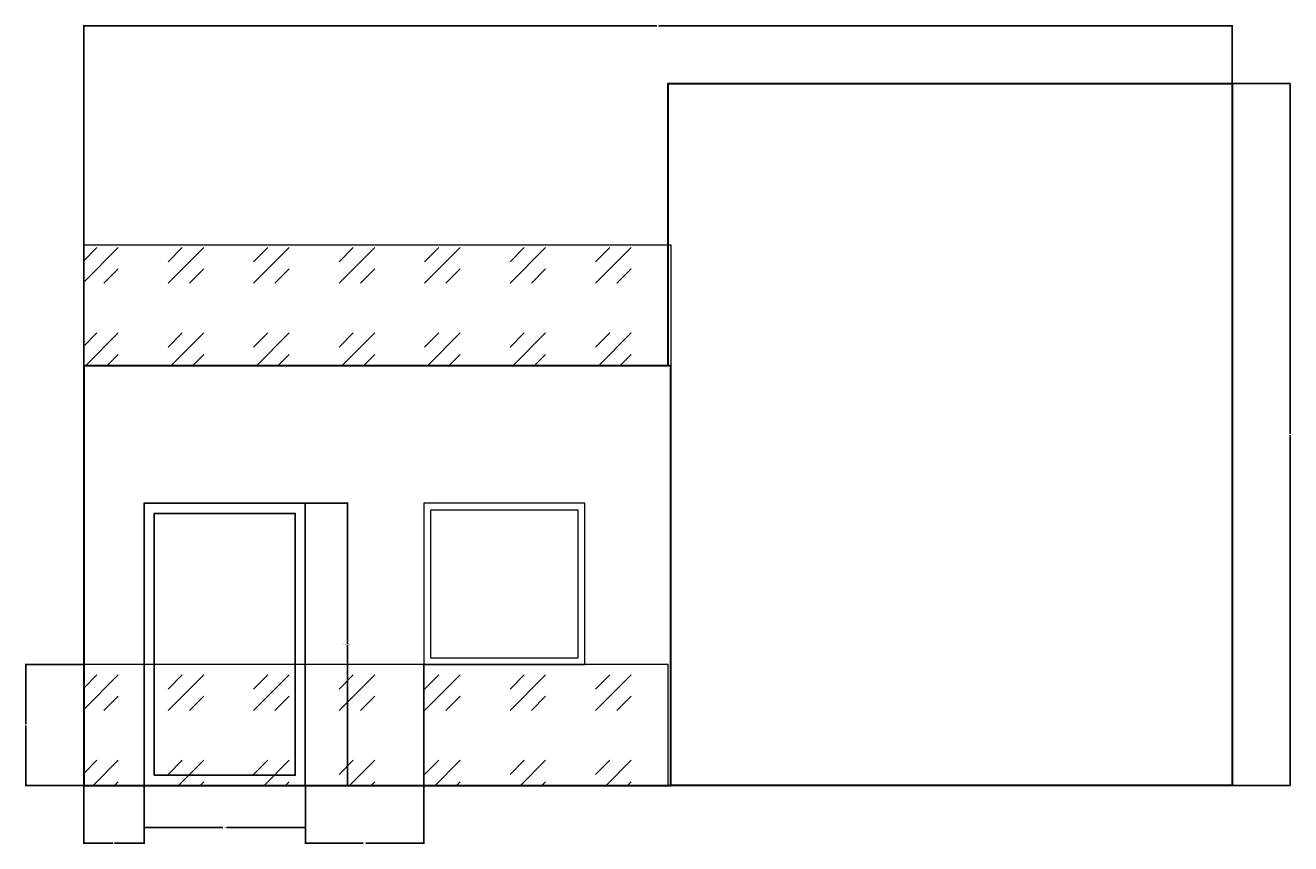
# Model space of a CAD drawing. Units: inches. Extents: x 810 to 2232, y 728 to 1827.
# Tile 3 of 6: x 1841 to 2218, y 749 to 993. Entities that reach past the tile are written whole.
import ezdxf

# ---------------------------------------------------------------- set-up
doc = ezdxf.new("R2010")
doc.units = ezdxf.units.IN
for name, color, linetype, lineweight in [('A-ANNO-DIMS', 2, 'Continuous', 18), ('A-ELEV', 7, 'Continuous', 30), ('A-ELEV-DOOR', 7, 'Continuous', 25), ('A-ELEV-GLAZ', 7, 'Continuous', 18), ('A-ELEV-PATT', 8, 'Continuous', 13)]:
    doc.layers.add(name, color=color, linetype=linetype, lineweight=lineweight)
doc.styles.get("Standard").update_dxf_attribs({"font": 'arial.ttf'})
doc.dimstyles.get("Standard").update_dxf_attribs({"dimtxt": 0.18, "dimasz": 0.18, "dimexe": 0.18, "dimexo": 0.0625, "dimgap": 0.09, "dimtad": 0, "dimtih": 1, "dimtoh": 1, "dimdec": 4, "dimzin": 0, "dimdsep": 46, "dimtxsty": 'Standard', "dimcen": 0.09, "dimadec": 0, "dimazin": 0, "dimtfac": 1, "dimtdec": 4, "dimtofl": 0, "dimtmove": 0, "dimatfit": 3, "dimfxl": 1, "dimtolj": 1, "dimtzin": 0, "dimarcsym": 0})

# ---------------------------------------------------------------- blocks, each defined once
blk = doc.blocks.new('DOOR-BALCONY-ELEV')
for points in [[(0, 0), (48, 0), (48, 84), (0, 84)], [(3, 3), (45, 3), (45, 81), (3, 81)]]:
    blk.add_lwpolyline(points, close=True)
blk = doc.blocks.new('WIN-ELEV-SQUARE')
for points in [[(0, 0), (48, 0), (48, 48), (0, 48)], [(2, 2), (46, 2), (46, 46), (2, 46)]]:
    blk.add_lwpolyline(points, close=True)
blk = doc.blocks.new('*D47')
at = {"layer": 'A-ANNO-DIMS', "color": 0, "lineweight": -2, "transparency": 16777216}
for p, q in [((1924.68, 850.84), (1937.4, 850.84)), ((1937.22, 850.66), (1937.22, 809.02)), ((1937.22, 767.02), (1937.22, 808.66)), ((1924.68, 766.84), (1937.4, 766.84))]:
    blk.add_line(p, q, dxfattribs=at)
at = {"layer": 'A-ANNO-DIMS', "color": 0, "transparency": 16777216}
for points in [[(1937.19, 850.66), (1937.25, 850.66), (1937.22, 850.84)], [(1937.19, 767.02), (1937.25, 767.02), (1937.22, 766.84)]]:
    blk.add_solid(points, dxfattribs=at)
at = {"layer": 'Defpoints', "color": 0, "transparency": 16777216}
for p in [(1924.62, 850.84), (1937.22, 850.84), (1924.62, 766.84)]:
    blk.add_point(p, dxfattribs=at)
at = {"layer": 'A-ANNO-DIMS', "color": 0, "transparency": 16777216, "insert": (1937.22, 808.84), "char_height": 0.18, "attachment_point": 5}
blk.add_mtext('\\A1;BALCONY DOOR 84 TYP.', dxfattribs=at)
blk = doc.blocks.new('*D48')
at = {"layer": 'A-ANNO-DIMS', "color": 0, "lineweight": -2, "transparency": 16777216}
for p, q in [((1876.62, 766.78), (1876.62, 754.06)), ((1924.62, 766.78), (1924.62, 754.06)), ((1876.8, 754.24), (1900.09, 754.24)), ((1924.44, 754.24), (1901.15, 754.24))]:
    blk.add_line(p, q, dxfattribs=at)
at = {"layer": 'A-ANNO-DIMS', "color": 0, "transparency": 16777216}
for points in [[(1876.8, 754.27), (1876.8, 754.21), (1876.62, 754.24)], [(1924.44, 754.27), (1924.44, 754.21), (1924.62, 754.24)]]:
    blk.add_solid(points, dxfattribs=at)
at = {"layer": 'Defpoints', "color": 0, "transparency": 16777216}
for p in [(1876.62, 766.84), (1924.62, 766.84), (1924.62, 754.24)]:
    blk.add_point(p, dxfattribs=at)
at = {"layer": 'A-ANNO-DIMS', "color": 0, "transparency": 16777216, "insert": (1900.62, 754.24), "char_height": 0.18, "attachment_point": 5}
blk.add_mtext('\\A1;48 TYP.', dxfattribs=at)
blk = doc.blocks.new('*D88')
at = {"layer": 'A-ANNO-DIMS', "color": 0, "lineweight": -2, "transparency": 16777216}
for p, q in [((1858.62, 766.9), (1858.62, 993.22)), ((1858.8, 993.04), (2029.33, 993.04)), ((2200.44, 993.04), (2029.9, 993.04)), ((2200.62, 766.9), (2200.62, 993.22))]:
    blk.add_line(p, q, dxfattribs=at)
at = {"layer": 'A-ANNO-DIMS', "color": 0, "transparency": 16777216}
for points in [[(1858.8, 993.07), (1858.8, 993.01), (1858.62, 993.04)], [(2200.44, 993.07), (2200.44, 993.01), (2200.62, 993.04)]]:
    blk.add_solid(points, dxfattribs=at)
at = {"layer": 'Defpoints', "color": 0, "transparency": 16777216}
for p in [(2200.62, 993.04), (1858.62, 766.84), (2200.62, 766.84)]:
    blk.add_point(p, dxfattribs=at)
at = {"layer": 'A-ANNO-DIMS', "color": 0, "transparency": 16777216, "insert": (2029.62, 993.04), "char_height": 0.18, "attachment_point": 5}
blk.add_mtext('\\A1;342', dxfattribs=at)
blk = doc.blocks.new('*D89')
at = {"layer": 'A-ANNO-DIMS', "color": 0, "lineweight": -2, "transparency": 16777216}
for p, q in [((2200.68, 975.84), (2218, 975.84)), ((2217.82, 975.66), (2217.82, 871.52)), ((2217.82, 767.02), (2217.82, 871.16)), ((2200.68, 766.84), (2218, 766.84))]:
    blk.add_line(p, q, dxfattribs=at)
at = {"layer": 'A-ANNO-DIMS', "color": 0, "transparency": 16777216}
for points in [[(2217.79, 975.66), (2217.85, 975.66), (2217.82, 975.84)], [(2217.79, 767.02), (2217.85, 767.02), (2217.82, 766.84)]]:
    blk.add_solid(points, dxfattribs=at)
at = {"layer": 'Defpoints', "color": 0, "transparency": 16777216}
for p in [(2200.62, 975.84), (2217.82, 975.84), (2200.62, 766.84)]:
    blk.add_point(p, dxfattribs=at)
at = {"layer": 'A-ANNO-DIMS', "color": 0, "transparency": 16777216, "insert": (2217.82, 871.34), "char_height": 0.18, "attachment_point": 5}
blk.add_mtext('\\A1;209', dxfattribs=at)
blk = doc.blocks.new('*D90')
at = {"layer": 'A-ANNO-DIMS', "color": 0, "lineweight": -2, "transparency": 16777216}
for p, q in [((1858.62, 766.78), (1858.62, 749.46)), ((1876.62, 766.78), (1876.62, 749.46)), ((1858.8, 749.64), (1867.41, 749.64)), ((1876.44, 749.64), (1867.83, 749.64))]:
    blk.add_line(p, q, dxfattribs=at)
at = {"layer": 'A-ANNO-DIMS', "color": 0, "transparency": 16777216}
for points in [[(1858.8, 749.67), (1858.8, 749.61), (1858.62, 749.64)], [(1876.44, 749.67), (1876.44, 749.61), (1876.62, 749.64)]]:
    blk.add_solid(points, dxfattribs=at)
at = {"layer": 'Defpoints', "color": 0, "transparency": 16777216}
for p in [(1858.62, 766.84), (1876.62, 766.84), (1876.62, 749.64)]:
    blk.add_point(p, dxfattribs=at)
at = {"layer": 'A-ANNO-DIMS', "color": 0, "transparency": 16777216, "insert": (1867.62, 749.64), "char_height": 0.18, "attachment_point": 5}
blk.add_mtext('\\A1;18', dxfattribs=at)
blk = doc.blocks.new('*D91')
at = {"layer": 'A-ANNO-DIMS', "color": 0, "lineweight": -2, "transparency": 16777216}
for p, q in [((1959.87, 802.78), (1959.87, 749.46)), ((1924.62, 766.78), (1924.62, 749.46)), ((1924.8, 749.64), (1941.85, 749.64)), ((1959.69, 749.64), (1942.64, 749.64))]:
    blk.add_line(p, q, dxfattribs=at)
at = {"layer": 'A-ANNO-DIMS', "color": 0, "transparency": 16777216}
for points in [[(1924.8, 749.67), (1924.8, 749.61), (1924.62, 749.64)], [(1959.69, 749.67), (1959.69, 749.61), (1959.87, 749.64)]]:
    blk.add_solid(points, dxfattribs=at)
at = {"layer": 'Defpoints', "color": 0, "transparency": 16777216}
for p in [(1959.87, 802.84), (1924.62, 766.84), (1959.87, 749.64)]:
    blk.add_point(p, dxfattribs=at)
at = {"layer": 'A-ANNO-DIMS', "color": 0, "transparency": 16777216, "insert": (1942.24, 749.64), "char_height": 0.18, "attachment_point": 5}
blk.add_mtext('\\A1;35.25', dxfattribs=at)
blk = doc.blocks.new('*D92')
at = {"layer": 'A-ANNO-DIMS', "color": 0, "lineweight": -2, "transparency": 16777216}
for p, q in [((1858.55, 802.84), (1841.24, 802.84)), ((1841.42, 802.66), (1841.42, 785.02)), ((1841.42, 767.02), (1841.42, 784.66)), ((1858.55, 766.84), (1841.24, 766.84))]:
    blk.add_line(p, q, dxfattribs=at)
at = {"layer": 'A-ANNO-DIMS', "color": 0, "transparency": 16777216}
for points in [[(1841.39, 802.66), (1841.45, 802.66), (1841.42, 802.84)], [(1841.39, 767.02), (1841.45, 767.02), (1841.42, 766.84)]]:
    blk.add_solid(points, dxfattribs=at)
at = {"layer": 'Defpoints', "color": 0, "transparency": 16777216}
for p in [(1841.42, 802.84), (1858.62, 802.84), (1858.62, 766.84)]:
    blk.add_point(p, dxfattribs=at)
at = {"layer": 'A-ANNO-DIMS', "color": 0, "transparency": 16777216, "insert": (1841.42, 784.84), "char_height": 0.18, "attachment_point": 5}
blk.add_mtext('\\A1;36', dxfattribs=at)

msp = doc.modelspace()

# ---------------------------------------------------------------- hatches: boundary and pattern name
at = {"layer": 'A-ELEV-PATT'}
h = msp.add_hatch(dxfattribs=at)
h.set_pattern_fill('GOST_GLASS', color=256, scale=3)
h.paths.add_polyline_path([(2033.4604, 891.8406), (1858.617, 891.8406), (1858.617, 927.8406), (2033.4604, 927.8406)])
h = msp.add_hatch(dxfattribs=at)
h.set_pattern_fill('GOST_GLASS', color=256, scale=3)
h.paths.add_polyline_path([(1858.617, 766.8406), (2032.617, 766.8406), (2032.617, 802.8406), (1858.617, 802.8406)])

# ---------------------------------------------------------------- linework, layer by layer
at = {"layer": 'A-ELEV'}
for points in [[(2033.4604, 891.8406), (2032.617, 891.8406), (2032.617, 975.8406), (2200.617, 975.8406), (2200.617, 891.8406)], [(2200.617, 927.8406), (2200.617, 891.8406)], [(2200.617, 891.8406), (2200.617, 766.8406), (2033.4604, 766.8406), (2033.4604, 891.8406)]]:
    msp.add_lwpolyline(points, dxfattribs=at)
msp.add_lwpolyline([(1858.617, 766.8406), (2033.4604, 766.8406), (2033.4604, 891.8406), (1858.617, 891.8406)], close=True, dxfattribs=at)
at = {"layer": 'A-ELEV-GLAZ'}
for points in [[(2033.4604, 891.8406), (1858.617, 891.8406), (1858.617, 927.8406), (2033.4604, 927.8406)], [(1858.617, 766.8406), (2032.617, 766.8406), (2032.617, 802.8406), (1858.617, 802.8406)]]:
    msp.add_lwpolyline(points, close=True, dxfattribs=at)

# ---------------------------------------------------------------- block references
at = {"layer": 'A-ELEV-DOOR'}
msp.add_blockref('DOOR-BALCONY-ELEV', (1876.617, 766.841), dxfattribs=at)
at = {"layer": 'A-ELEV-GLAZ'}
msp.add_blockref('WIN-ELEV-SQUARE', (1959.867, 802.841), dxfattribs=at)

# ---------------------------------------------------------------- dimensions: what is measured, and where the dimension line sits
at = {"layer": 'A-ANNO-DIMS'}
for base, p1, p2, override, picture, middle in [((2200.617, 993.0406), (1858.617, 766.8406), (2200.617, 766.8406), {"dimdec": 0, "dimlfac": 1, "dimrnd": 0, "dimzin": 0, "dimdsep": 46, "dimlunit": 2}, '*D88', (2029.617, 993.0406)), ((1959.867, 749.6406), (1924.617, 766.8406), (1959.867, 802.8406), {"dimdec": 2, "dimlfac": 1, "dimrnd": 0, "dimzin": 0, "dimdsep": 46, "dimlunit": 2}, '*D91', (1942.242, 749.6406)), ((1876.617, 749.6406), (1858.617, 766.8406), (1876.617, 766.8406), {"dimdec": 0, "dimlfac": 1, "dimrnd": 0, "dimzin": 0, "dimdsep": 46, "dimlunit": 2}, '*D90', (1867.617, 749.6406))]:
    dim = msp.add_linear_dim(base=base, p1=p1, p2=p2, dimstyle='Standard', override=override, dxfattribs=at)
    dim.commit()
    dim.dimension.update_dxf_attribs({"geometry": picture, "text_midpoint": middle})
for base, p1, p2, picture, middle in [((2217.817, 975.8406), (2200.617, 766.8406), (2200.617, 975.8406), '*D89', (2217.817, 871.3406)), ((1841.417, 802.8406), (1858.617, 766.8406), (1858.617, 802.8406), '*D92', (1841.417, 784.8406))]:
    dim = msp.add_linear_dim(base=base, p1=p1, p2=p2, angle=90, dimstyle='Standard', override={"dimdec": 0, "dimlfac": 1, "dimrnd": 0, "dimzin": 0, "dimdsep": 46, "dimlunit": 2}, dxfattribs=at)
    dim.commit()
    dim.dimension.update_dxf_attribs({"geometry": picture, "text_midpoint": middle})
dim = msp.add_linear_dim(base=(1937.217, 850.8406), p1=(1924.617, 766.8406), p2=(1924.617, 850.8406), angle=90, text='BALCONY DOOR <> TYP.', dimstyle='Standard', override={"dimdec": 0, "dimlfac": 1, "dimrnd": 0, "dimzin": 0, "dimdsep": 46, "dimlunit": 2}, dxfattribs=at)
dim.commit()
dim.dimension.update_dxf_attribs({"geometry": '*D47', "text_midpoint": (1937.217, 808.8406)})
dim = msp.add_linear_dim(base=(1924.617, 754.2406), p1=(1876.617, 766.8406), p2=(1924.617, 766.8406), text='<> TYP.', dimstyle='Standard', override={"dimdec": 0, "dimlfac": 1, "dimrnd": 0, "dimzin": 0, "dimdsep": 46, "dimlunit": 2}, dxfattribs=at)
dim.commit()
dim.dimension.update_dxf_attribs({"geometry": '*D48', "text_midpoint": (1900.617, 754.2406)})

doc.saveas('drawing.dxf')
